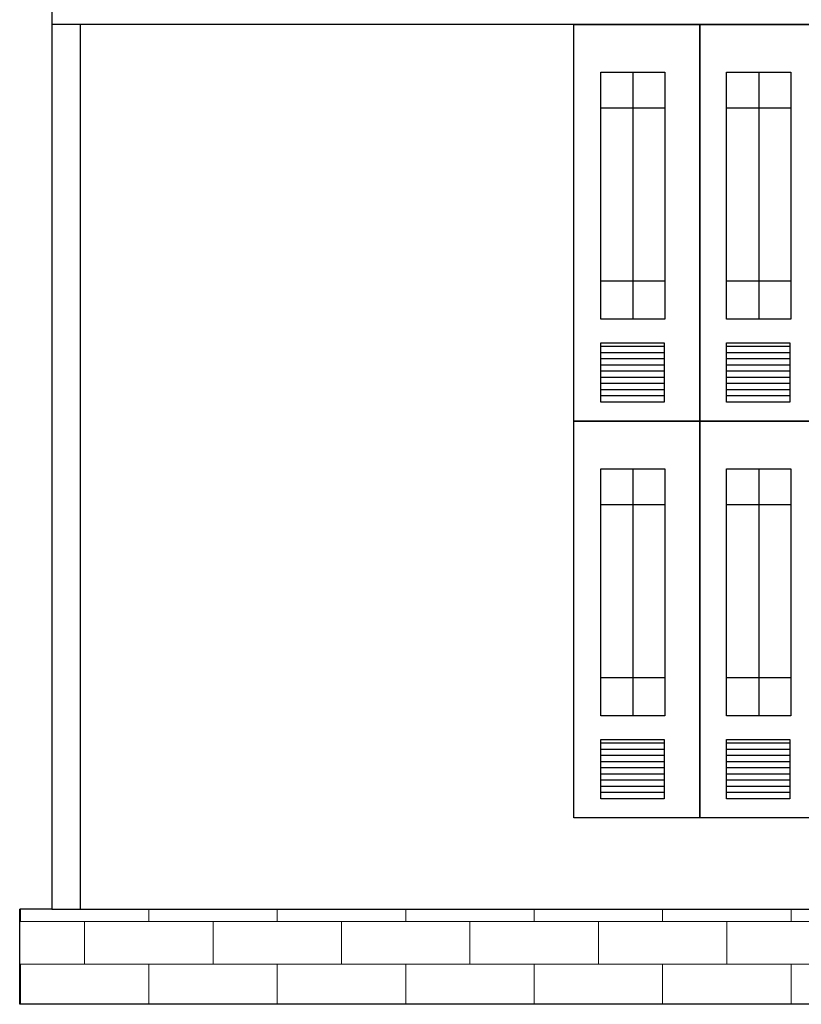
# Model space of a CAD drawing. Units: metres. Extents: x 10365 to 12529, y 3661 to 6248.
# Tile 3 of 9: x 10574 to 10987, y 4875 to 5397. Entities that reach past the tile are written whole.
import ezdxf

# ---------------------------------------------------------------- set-up
doc = ezdxf.new("R2010")
doc.units = ezdxf.units.M
doc.header["$MEASUREMENT"] = 0
doc.layers.add('A-ELEV', color=7, linetype='Continuous', lineweight=25)
doc.layers.add('A-ELEV-PATT', color=8, linetype='Continuous', lineweight=13)

msp = doc.modelspace()

# ---------------------------------------------------------------- hatches: boundary and pattern name
at = {"layer": 'A-ELEV-PATT'}
h = msp.add_hatch(dxfattribs=at)
h.set_pattern_fill('AR-BRSTD', color=256, scale=8.5)
h.paths.add_polyline_path([(11113.98, 4925.82), (10590.74, 4925.82), (10573.67, 4925.82), (10573.67, 4875.44), (11113.98, 4875.44)])

# ---------------------------------------------------------------- linework, layer by layer
at = {"layer": 'A-ELEV'}
for p, q in [((11343.22, 5394.05), (10590.74, 5394.05)), ((10898.31, 5368.73), (10898.31, 5238.09)), ((10964.91, 5368.73), (10964.91, 5238.09)), ((10881.34, 5349.84), (10915.29, 5349.84)), ((10947.94, 5349.84), (10981.89, 5349.84)), ((10881.34, 5258.3), (10915.29, 5258.3)), ((10947.94, 5258.3), (10981.89, 5258.3)), ((10881.34, 5223.7), (10914.77, 5223.7)), ((10947.94, 5223.7), (10981.38, 5223.7)), ((10881.34, 5220.44), (10914.77, 5220.44)), ((10881.34, 5217.18), (10914.77, 5217.18)), ((10947.94, 5220.44), (10981.38, 5220.44)), ((10947.94, 5217.18), (10981.38, 5217.18)), ((10881.34, 5213.92), (10914.77, 5213.92)), ((10947.94, 5213.92), (10981.38, 5213.92)), ((10881.34, 5210.66), (10914.77, 5210.66)), ((10881.34, 5207.4), (10914.77, 5207.4)), ((10947.94, 5210.66), (10981.38, 5210.66)), ((10947.94, 5207.4), (10981.38, 5207.4)), ((10881.34, 5204.13), (10914.77, 5204.13)), ((10881.34, 5204.13), (10914.77, 5204.13)), ((10881.34, 5200.87), (10914.77, 5200.87)), ((10947.94, 5204.13), (10981.38, 5204.13)), ((10947.94, 5204.13), (10981.38, 5204.13)), ((10947.94, 5200.87), (10981.38, 5200.87)), ((10881.34, 5197.61), (10914.77, 5197.61)), ((10947.94, 5197.61), (10981.38, 5197.61)), ((10898.31, 5158.81), (10898.31, 5028.16)), ((10964.91, 5158.81), (10964.91, 5028.16)), ((10881.34, 5139.92), (10915.29, 5139.92)), ((10947.94, 5139.92), (10981.89, 5139.92)), ((10881.34, 5048.38), (10915.29, 5048.38)), ((10947.94, 5048.38), (10981.89, 5048.38)), ((10881.34, 5013.78), (10914.77, 5013.78)), ((10947.94, 5013.78), (10981.38, 5013.78)), ((10881.34, 5010.52), (10914.77, 5010.52)), ((10947.94, 5010.52), (10981.38, 5010.52)), ((10881.34, 5007.26), (10914.77, 5007.26)), ((10881.34, 5003.99), (10914.77, 5003.99)), ((10947.94, 5007.26), (10981.38, 5007.26)), ((10947.94, 5003.99), (10981.38, 5003.99)), ((10881.34, 5000.73), (10914.77, 5000.73)), ((10881.34, 4997.47), (10914.77, 4997.47)), ((10947.94, 5000.73), (10981.38, 5000.73)), ((10947.94, 4997.47), (10981.38, 4997.47)), ((10881.34, 4994.21), (10914.77, 4994.21)), ((10881.34, 4994.21), (10914.77, 4994.21)), ((10947.94, 4994.21), (10981.38, 4994.21)), ((10947.94, 4994.21), (10981.38, 4994.21)), ((10881.34, 4990.95), (10914.77, 4990.95)), ((10881.34, 4987.69), (10914.77, 4987.69)), ((10947.94, 4990.95), (10981.38, 4990.95)), ((10947.94, 4987.69), (10981.38, 4987.69)), ((10605.74, 4940.82), (10605.74, 4925.82)), ((10573.67, 4875.44), (10573.67, 4925.82)), ((10590.74, 4925.82), (10573.67, 4925.82)), ((11343.22, 4875.44), (10573.67, 4875.44))]:
    msp.add_line(p, q, dxfattribs=at)
for points in [[(11343.22, 5554.17), (11343.22, 5554.17), (10590.74, 5554.17), (10590.74, 5554.17), (10590.74, 4925.82), (10590.74, 4925.82), (11343.22, 4925.82), (11343.22, 4925.82)], [(10867.07, 5394.05), (10867.07, 5394.05), (10933.68, 5394.05), (10933.68, 5394.05), (10933.68, 5184.13), (10933.68, 5184.13), (10867.07, 5184.13), (10867.07, 5184.13)], [(10933.68, 5394.05), (10933.68, 5394.05), (11000.28, 5394.05), (11000.28, 5394.05), (11000.28, 5184.13), (11000.28, 5184.13), (10933.68, 5184.13), (10933.68, 5184.13)], [(10881.34, 5368.73), (10881.34, 5368.73), (10915.29, 5368.73), (10915.29, 5368.73), (10915.29, 5238.09), (10915.29, 5238.09), (10881.34, 5238.09), (10881.34, 5238.09)], [(10947.94, 5368.73), (10947.94, 5368.73), (10981.89, 5368.73), (10981.89, 5368.73), (10981.89, 5238.09), (10981.89, 5238.09), (10947.94, 5238.09), (10947.94, 5238.09)], [(10881.34, 5225.53), (10881.34, 5225.53), (10914.77, 5225.53), (10914.77, 5225.53), (10914.77, 5194.04), (10914.77, 5194.04), (10881.34, 5194.04), (10881.34, 5194.04)], [(10947.94, 5225.53), (10947.94, 5225.53), (10981.38, 5225.53), (10981.38, 5225.53), (10981.38, 5194.04), (10981.38, 5194.04), (10947.94, 5194.04), (10947.94, 5194.04)], [(10867.07, 5184.13), (10867.07, 5184.13), (10933.68, 5184.13), (10933.68, 5184.13), (10933.68, 4974.2), (10933.68, 4974.2), (10867.07, 4974.2), (10867.07, 4974.2)], [(10933.68, 5184.13), (10933.68, 5184.13), (11000.28, 5184.13), (11000.28, 5184.13), (11000.28, 4974.2), (11000.28, 4974.2), (10933.68, 4974.2), (10933.68, 4974.2)], [(10881.34, 5158.81), (10881.34, 5158.81), (10915.29, 5158.81), (10915.29, 5158.81), (10915.29, 5028.16), (10915.29, 5028.16), (10881.34, 5028.16), (10881.34, 5028.16)], [(10947.94, 5158.81), (10947.94, 5158.81), (10981.89, 5158.81), (10981.89, 5158.81), (10981.89, 5028.16), (10981.89, 5028.16), (10947.94, 5028.16), (10947.94, 5028.16)], [(10881.34, 5015.6), (10881.34, 5015.6), (10914.77, 5015.6), (10914.77, 5015.6), (10914.77, 4984.11), (10914.77, 4984.11), (10881.34, 4984.11), (10881.34, 4984.11)], [(10947.94, 5015.6), (10947.94, 5015.6), (10981.38, 5015.6), (10981.38, 5015.6), (10981.38, 4984.11), (10981.38, 4984.11), (10947.94, 4984.11), (10947.94, 4984.11)]]:
    msp.add_lwpolyline(points, close=True, dxfattribs=at)
msp.add_lwpolyline([(10605.74, 5394.05), (10605.74, 4940.82)], dxfattribs=at)

doc.saveas('drawing.dxf')
